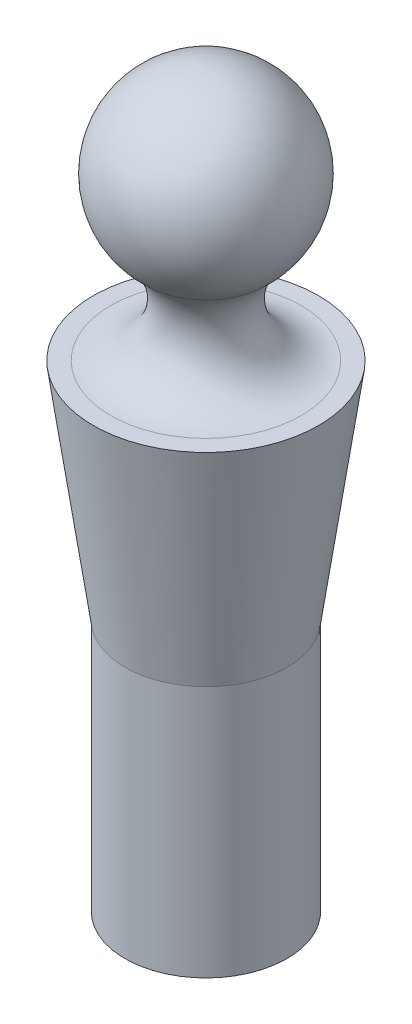
from build123d import *


with BuildPart() as part:
    # Pin Profile Sketch → Pin Body Revolve (revolve)
    with BuildSketch(Plane.XY, mode=Mode.PRIVATE) as pin_body_revolve_sk:
        with BuildLine():
            Line((9, 4.661084251), (12.5, 29.661084251))
            Line((12.5, 29.661084251), (10.583005244, 29.661084251))
            ThreePointArc((10.583005244, 29.661084251), (4.970519164, 33.539763908), (6.614378278, 40.161084251))
            ThreePointArc((6.614378278, 40.161084251), (9.354143467, 51.196618157), (0, 57.661084251))
            Line((0, 57.661084251), (0, 29.661084251))
            Line((0, 29.661084251), (0, 0))
            Line((0, 0), (0, -23.338915749))
            Line((0, -23.338915749), (9, -23.338915749))
            Line((9, -23.338915749), (9, 4.661084251))
        make_face()
    revolve(pin_body_revolve_sk.sketch.rotate(Axis((0, 0, 0), (0, 1, 0)), 90), axis=Axis((0, 0, 0), (0, 1, 0)))


solid = part.part
